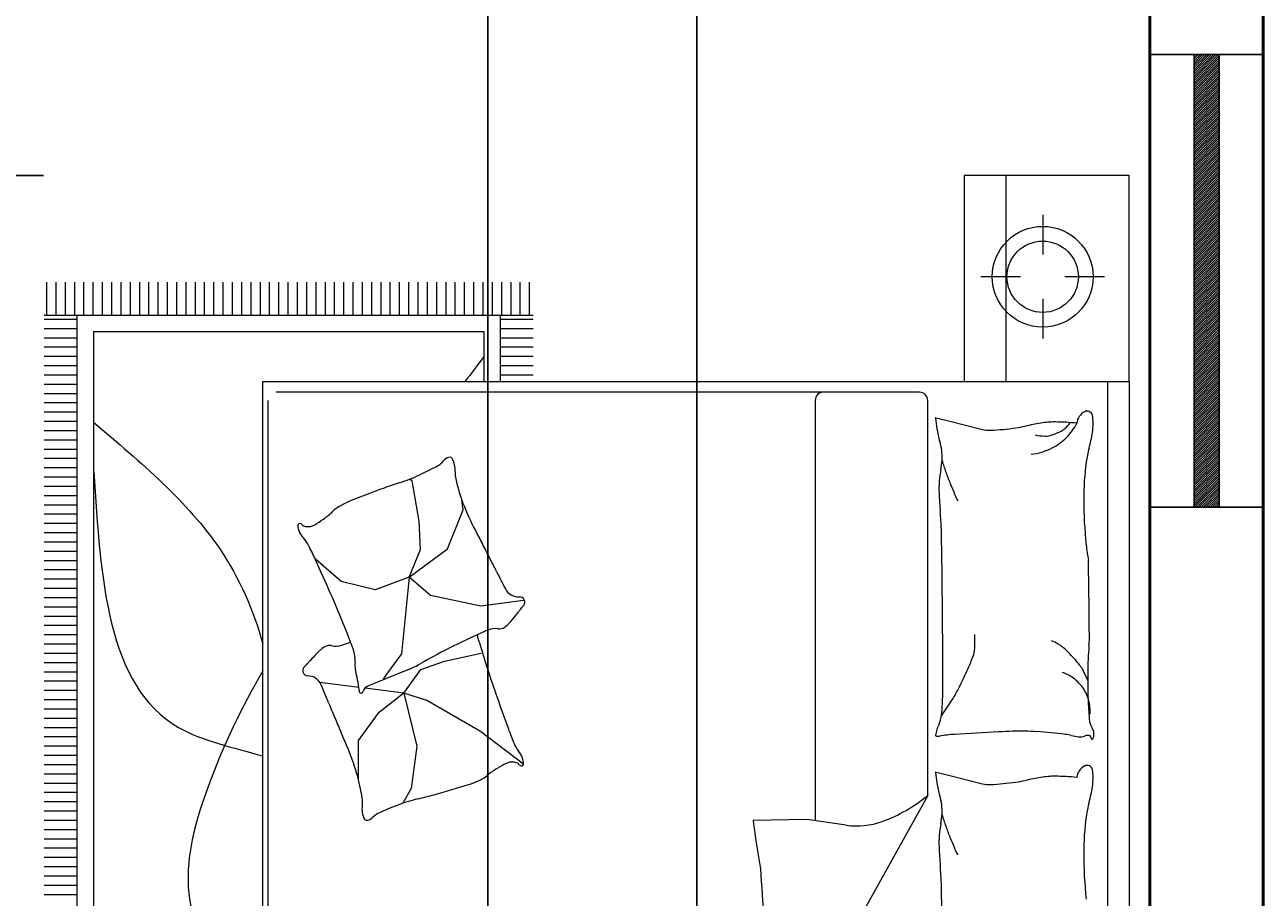
# Model space of a CAD drawing. Units: inches. Extents: x 338 to 1188, y -996 to 127.
# Tile 11 of 15: x 859 to 957, y -552 to -483. Entities that reach past the tile are written whole.
import ezdxf

# ---------------------------------------------------------------- set-up
doc = ezdxf.new("R2010")
doc.units = ezdxf.units.IN
doc.header["$MEASUREMENT"] = 0
for name, color, linetype, lineweight in [('A-ANNO-DIMS', 5, 'Continuous', 18), ('A-GLAZ-PATT', 5, 'Continuous', 13), ('wall', 1, 'Continuous', 50), ('win', 5, 'Continuous', 25)]:
    doc.layers.add(name, color=color, linetype=linetype, lineweight=lineweight)
doc.layers.add('furniture', color=50, linetype='Continuous', lineweight=13, transparency=0.8)
doc.styles.add('DIM_FONT', font='SIMPLEX.shx', dxfattribs={"width": 0.8})
doc.styles.get("Standard").update_dxf_attribs({"font": 'arial.ttf'})
doc.dimstyles.get("Standard").update_dxf_attribs({"dimtxt": 0.18, "dimasz": 0.18, "dimexe": 0.18, "dimexo": 0.0625, "dimgap": 0.09, "dimtad": 0, "dimtih": 1, "dimtoh": 1, "dimdec": 1, "dimzin": 0, "dimdsep": 46, "dimlunit": 4, "dimtxsty": 'Standard', "dimcen": 0.09, "dimadec": 0, "dimazin": 0, "dimtfac": 1, "dimtdec": 1, "dimtofl": 0, "dimtmove": 0, "dimatfit": 3, "dimfxl": 1, "dimtolj": 1, "dimtzin": 0, "dimarcsym": 0})

# ---------------------------------------------------------------- blocks, each defined once
blk = doc.blocks.new('A$C4F634EDD')
for p, q in [((0, 2.6295), (0, 2.2295)), ((0.5, 2.6295), (0, 2.6295)), ((0.5, 2.6295), (2.3, 2.6295)), ((0.5, 0.5295), (0.5, 2.6295)), ((0.5, 2.2295), (0.5, 2.6295)), ((0.2457, 2.5697), (0.2457, 2.4733)), ((0.5, 2.5771), (2.3, 2.5771)), ((0.0957, 2.4197), (0.192, 2.4197)), ((0.2994, 2.4197), (0.3957, 2.4197)), ((0.2457, 2.366), (0.2457, 2.2697)), ((0, 2.3301), (0.5, 2.3301)), ((0.5953, 2.1912), (0.616, 2.2738)), ((1.4546, 2.1912), (1.4752, 2.2738)), ((0, 2.2295), (0.5, 2.2295)), ((0.5878, 2.1612), (0.5953, 2.1912)), ((1.4471, 2.1612), (1.4546, 2.1912)), ((1.5035, 2.141), (0.5458, 2.141)), ((1.5035, 2.141), (2.2716, 1.7136)), ((0.5258, 2.121), (0.5258, 0.5617)), ((1.576, 1.9433), (1.5624, 1.8479)), ((0.5458, 1.8684), (1.5653, 1.8684)), ((1.5624, 1.8479), (1.5641, 1.7178)), ((0.2586, 1.1753), (0.3386, 1.1753)), ((0.3386, 0), (0.3386, 1.1852)), ((0.3486, 1.1052), (0.3486, 1.1852)), ((0.3711, 1.1052), (0.3711, 1.1852)), ((0.3936, 1.1052), (0.3936, 1.1852)), ((0.4161, 1.1052), (0.4161, 1.1852)), ((0.4386, 1.1052), (0.4386, 1.1852)), ((0.4611, 1.1052), (0.4611, 1.1852)), ((0.4836, 1.1052), (0.4836, 1.1852)), ((0.2586, 1.1528), (0.3386, 1.1528)), ((1.031, 1.1612), (1.0448, 1.0581)), ((1.4276, 1.1611), (1.3484, 1.0571)), ((0.2586, 1.1303), (0.3386, 1.1303)), ((0.2586, 1.1078), (0.3386, 1.1078)), ((0.2586, 1.0853), (0.3386, 1.0853)), ((0.3386, 1.1052), (0.5, 1.1052)), ((0.2586, 1.0628), (0.3386, 1.0628)), ((0.3786, 1.0652), (0.5, 1.0652)), ((0.3786, 0.12), (0.3786, 1.0652)), ((1.0448, 1.0581), (1.019, 0.936)), ((1.1784, 0.9702), (1.1586, 1.0591)), ((1.3484, 1.0571), (1.2733, 0.9268)), ((0.2586, 1.0403), (0.3386, 1.0403)), ((0.2586, 1.0178), (0.3386, 1.0178)), ((0.2586, 0.9953), (0.3386, 0.9953)), ((0.8108, 1.0151), (0.7868, 1.0117)), ((0.9054, 0.9773), (0.8108, 1.0151)), ((0.2586, 0.9728), (0.3386, 0.9728)), ((0.9743, 0.8845), (0.9054, 0.9773)), ((1.1982, 0.9129), (1.1784, 0.9702)), ((0.2586, 0.9503), (0.3386, 0.9503)), ((1.019, 0.936), (0.9743, 0.8845)), ((0.2586, 0.9278), (0.3386, 0.9278)), ((0.2586, 0.9053), (0.3386, 0.9053)), ((0.8384, 0.9085), (0.7403, 0.8913)), ((0.9072, 0.912), (0.8384, 0.9085)), ((0.9743, 0.8845), (0.9072, 0.912)), ((1.2555, 0.8715), (1.1982, 0.9129)), ((1.2733, 0.9268), (1.2555, 0.8715)), ((1.2555, 0.8715), (1.384, 0.9031)), ((1.384, 0.9031), (1.4868, 0.8892)), ((0.2586, 0.8828), (0.3386, 0.8828)), ((0.7403, 0.8913), (0.737, 0.8849)), ((0.9743, 0.8845), (1.0052, 0.802)), ((0.9743, 0.8845), (1.16, 0.8656)), ((1.1973, 0.8853), (1.2203, 0.829)), ((1.2555, 0.8715), (1.2437, 0.7773)), ((1.2555, 0.8715), (1.3049, 0.8082)), ((1.4868, 0.8892), (1.5228, 0.8692)), ((0.2586, 0.8603), (0.3386, 0.8603)), ((1.16, 0.8656), (1.2099, 0.8295)), ((0.2586, 0.8378), (0.3386, 0.8378)), ((0.2586, 0.8153), (0.3386, 0.8153)), ((1.2099, 0.8295), (1.222, 0.8209)), ((1.2203, 0.829), (1.2381, 0.7855)), ((0.2586, 0.7928), (0.3386, 0.7928)), ((1.0052, 0.802), (0.9846, 0.7194)), ((1.3049, 0.8082), (1.3701, 0.7608)), ((0.2586, 0.7703), (0.3386, 0.7703)), ((1.2419, 0.7626), (1.23, 0.668)), ((1.3701, 0.7608), (1.463, 0.7608)), ((0.2586, 0.7478), (0.3386, 0.7478)), ((0.2586, 0.7253), (0.3386, 0.7253)), ((0.2586, 0.7028), (0.3386, 0.7028)), ((0.9846, 0.7194), (0.931, 0.6569)), ((0.2586, 0.6803), (0.3386, 0.6803)), ((0.2586, 0.6578), (0.3386, 0.6578)), ((0.2586, 0.6353), (0.3386, 0.6353)), ((0.2586, 0.6128), (0.3386, 0.6128)), ((0.2586, 0.5903), (0.3386, 0.5903)), ((0.2586, 0.5678), (0.3386, 0.5678)), ((0.2586, 0.5453), (0.3386, 0.5453)), ((0.5458, 0.5417), (2.2516, 0.5417)), ((0.2586, 0.5228), (0.3386, 0.5228)), ((2.3, 0.5295), (0.5, 0.5295)), ((0.2586, 0.5003), (0.3386, 0.5003)), ((0.2586, 0.4778), (0.3386, 0.4778)), ((0.2586, 0.4553), (0.3386, 0.4553)), ((0.2586, 0.4328), (0.3386, 0.4328)), ((0.2586, 0.4103), (0.3386, 0.4103)), ((0.2586, 0.3878), (0.3386, 0.3878)), ((0.2586, 0.3653), (0.3386, 0.3653)), ((0.2586, 0.3428), (0.3386, 0.3428)), ((0.2586, 0.3203), (0.3386, 0.3203)), ((0.2586, 0.2978), (0.3386, 0.2978)), ((0.2586, 0.2753), (0.3386, 0.2753)), ((0.2586, 0.2528), (0.3386, 0.2528)), ((0.2586, 0.2303), (0.3386, 0.2303)), ((0.2586, 0.2078), (0.3386, 0.2078)), ((0.2586, 0.1853), (0.3386, 0.1853)), ((0.2586, 0.1628), (0.3386, 0.1628)), ((0.2586, 0.1403), (0.3386, 0.1403)), ((0.2586, 0.1178), (0.3386, 0.1178)), ((0.2586, 0.0953), (0.3386, 0.0953)), ((2.4188, 0.12), (0.3786, 0.12)), ((0.2586, 0.0728), (0.3386, 0.0728)), ((2.4588, 0.08), (0.3386, 0.08)), ((0.3486, 0), (0.3486, 0.08)), ((0.3711, 0), (0.3711, 0.08)), ((0.3936, 0), (0.3936, 0.08)), ((0.4161, 0), (0.4161, 0.08)), ((0.4386, 0), (0.4386, 0.08)), ((0.4611, 0), (0.4611, 0.08)), ((0.4836, 0), (0.4836, 0.08)), ((0.5061, 0), (0.5061, 0.08)), ((0.5286, 0), (0.5286, 0.08)), ((0.5511, 0), (0.5511, 0.08)), ((0.5736, 0), (0.5736, 0.08)), ((0.5961, 0), (0.5961, 0.08)), ((0.6186, 0), (0.6186, 0.08)), ((0.6411, 0), (0.6411, 0.08)), ((0.6636, 0), (0.6636, 0.08)), ((0.6861, 0), (0.6861, 0.08)), ((0.7086, 0), (0.7086, 0.08)), ((0.7311, 0), (0.7311, 0.08)), ((0.7536, 0), (0.7536, 0.08)), ((0.7761, 0), (0.7761, 0.08)), ((0.7986, 0), (0.7986, 0.08)), ((0.8211, 0), (0.8211, 0.08)), ((0.8436, 0), (0.8436, 0.08)), ((0.8661, 0), (0.8661, 0.08)), ((0.8886, 0), (0.8886, 0.08)), ((0.9111, 0), (0.9111, 0.08)), ((0.9336, 0), (0.9336, 0.08)), ((0.9561, 0), (0.9561, 0.08)), ((0.9786, 0), (0.9786, 0.08)), ((1.0011, 0), (1.0011, 0.08)), ((1.0236, 0), (1.0236, 0.08)), ((1.0461, 0), (1.0461, 0.08)), ((1.0686, 0), (1.0686, 0.08)), ((1.0911, 0), (1.0911, 0.08)), ((1.1136, 0), (1.1136, 0.08)), ((1.1361, 0), (1.1361, 0.08)), ((1.1586, 0), (1.1586, 0.08)), ((1.1811, 0), (1.1811, 0.08)), ((1.2036, 0), (1.2036, 0.08)), ((1.2261, 0), (1.2261, 0.08)), ((1.2486, 0), (1.2486, 0.08)), ((1.2711, 0), (1.2711, 0.08)), ((1.2936, 0), (1.2936, 0.08)), ((1.3161, 0), (1.3161, 0.08)), ((1.3386, 0), (1.3386, 0.08)), ((1.3611, 0), (1.3611, 0.08)), ((1.3836, 0), (1.3836, 0.08)), ((1.4061, 0), (1.4061, 0.08)), ((1.4286, 0), (1.4286, 0.08)), ((1.4511, 0), (1.4511, 0.08)), ((1.4736, 0), (1.4736, 0.08)), ((1.4961, 0), (1.4961, 0.08)), ((1.5186, 0), (1.5186, 0.08)), ((1.5411, 0), (1.5411, 0.08)), ((1.5636, 0), (1.5636, 0.08)), ((1.5861, 0), (1.5861, 0.08)), ((1.6086, 0), (1.6086, 0.08)), ((1.6311, 0), (1.6311, 0.08)), ((1.6536, 0), (1.6536, 0.08)), ((1.6761, 0), (1.6761, 0.08)), ((1.6986, 0), (1.6986, 0.08)), ((1.7211, 0), (1.7211, 0.08)), ((1.7436, 0), (1.7436, 0.08)), ((0.2586, 0.0503), (0.3386, 0.0503)), ((0.2586, 0.0278), (0.3386, 0.0278)), ((0.2586, 0.0053), (0.3386, 0.0053))]:
    blk.add_line(p, q)
for radius in [0.1222, 0.0865]:
    blk.add_circle((0.2457, 2.4197), radius)
for centre, radius, start, end in [((0.5848, 2.5274), 0.0131, 101.2724, 206.5805), ((0.6036, 2.5368), 0.0342, 206.5805, 265.5998), ((0.5999, 2.4516), 0.0904, 90, 101.2724), ((0.5999, 2.3808), 0.1611, 81.5628, 90), ((0.5788, 2.2388), 0.3048, 74.256, 81.5628), ((0.7272, 2.7653), 0.2422, 254.256, 262.4531), ((0.7851, 3.2019), 0.6827, 262.4531, 270), ((0.7851, 3.5682), 1.049, 270, 276.0867), ((0.8402, 3.0514), 0.5293, 276.0867, 280.1899), ((1.1602, -8.1346), 10.6675, 90.30153, 91.21582), ((1.1169, 2.2433), 0.2897, 85.1982, 92.5386), ((1.2142, 3.4021), 0.8732, 265.1982, 269.4243), ((1.3082, 2.3102), 0.234, 110.8603, 117.2396), ((1.2204, 4.0232), 1.4943, 269.4243, 271.9079), ((1.2995, 2.4357), 0.0992, 105.9352, 126.0864), ((1.2429, 3.3501), 0.8208, 271.9079, 275.2592), ((1.2995, 2.4357), 0.0992, 85.7841, 105.9352), ((1.3132, 2.5864), 0.0539, 275.2592, 300.6513), ((1.3554, 2.5152), 0.0289, 85.6975, 120.6513), ((1.3556, 2.519), 0.0251, 68.2117, 85.6975), ((1.3739, 2.5288), 0.0156, 158.0096, 201.421), ((1.3634, 2.533), 0.00428, 78.1069, 158.0096), ((1.3288, 2.5111), 0.0328, 351.8665, 21.421), ((1.3647, 2.5395), 0.00232, 258.1069, 19.564), ((1.3637, 2.5391), 0.00342, 19.564, 68.2117), ((1.444, 2.5274), 0.0131, 101.2724, 206.5805), ((1.4628, 2.5368), 0.0342, 206.5805, 265.5998), ((1.4591, 2.4516), 0.0904, 90, 101.2724), ((1.4591, 2.3808), 0.1611, 81.5628, 90), ((1.438, 2.2388), 0.3048, 74.256, 81.5628), ((1.5865, 2.7653), 0.2422, 254.256, 262.4531), ((1.6443, 3.2019), 0.6827, 262.4531, 270), ((1.6443, 3.5682), 1.049, 270, 276.0867), ((1.0898, 2.4496), 0.4918, 173.7676, 180), ((0.5368, 2.3783), 0.1399, 45.0976, 62.7964), ((1.4317, 2.2032), 0.3916, 128.3886, 133.8115), ((1.2362, 2.45), 0.0768, 117.2396, 128.3886), ((1.2995, 2.4357), 0.0992, 143.8234, 161.5603), ((1.2995, 2.4357), 0.0992, 126.0864, 143.8234), ((1.1177, 2.5413), 0.246, 347.8905, 351.8665), ((1.949, 2.4496), 0.4918, 173.7676, 180), ((0.5462, 2.4142), 0.0899, 41.4429, 53.7359), ((0.5741, 2.4389), 0.0526, 25.3551, 41.4429), ((0.4851, 2.3967), 0.1511, 21.8149, 25.3551), ((0.5368, 2.3783), 0.1399, 27.3988, 45.0976), ((1.1799, 2.4341), 0.0493, 140.9651, 151.6832), ((1.3165, 2.3233), 0.2252, 133.8115, 140.9651), ((2.2605, 2.3525), 0.9131, 172.3191, 176.6313), ((1.5522, 2.448), 0.1983, 167.8905, 172.3191), ((0.8019, 2.4496), 0.204, 180, 189.6844), ((0.4345, 2.3765), 0.2056, 18.7799, 21.8149), ((0.576, 2.4246), 0.0562, 0, 18.7799), ((0.5368, 2.3783), 0.1399, 16.515, 27.3988), ((1.3127, 2.3625), 0.2002, 151.6832, 156.9972), ((1.6611, 2.4496), 0.204, 180, 189.6844), ((1.4703, 2.5637), 0.882, 189.6844, 192.1984), ((0.5406, 2.4246), 0.0915, 345.3149, 0), ((0.5368, 2.3783), 0.1399, 5.6311, 16.515), ((2.0266, 2.3663), 0.6787, 176.6313, 181.6331), ((2.3295, 2.5637), 0.882, 189.6844, 192.1984), ((0.2982, 2.3103), 0.3171, 8.0051, 12.1984), ((1.1575, 2.3103), 0.3171, 8.0051, 12.1984), ((-0.0401, 2.2627), 0.6588, 2.6649, 8.0051), ((2.7128, 2.3859), 1.3652, 181.6331, 183.055), ((0.8191, 2.2627), 0.6588, 2.6649, 8.0051), ((14.9657, 3.0398), 13.6356, 183.05496, 183.50486), ((0.5503, 2.2902), 0.0677, 345.9548, 2.6649), ((1.4096, 2.2902), 0.0677, 345.9548, 2.6649), ((1.1303, 1.9835), 0.2721, 85.9172, 93.5552), ((1.1455, 2.197), 0.058, 69.3257, 85.9172), ((0.9871, 1.7772), 0.5066, 65.6735, 69.3257), ((0.6058, 0.9338), 1.4323, 63.5015, 65.6735), ((0.473, 2.8815), 0.7387, 289.428, 291.6577), ((0.473, 2.8815), 0.7387, 291.6577, 293.4844), ((0.473, 2.8815), 0.7387, 293.4844, 295.3111), ((1.1054, 1.9358), 0.3126, 57.865, 63.5015), ((0.8841, 1.5835), 0.7286, 54.1737, 57.865), ((1.6762, 2.2258), 0.3212, 183.5049, 189.9984), ((1.3322, 2.8815), 0.7387, 289.428, 291.6577), ((1.3322, 2.8815), 0.7387, 291.6577, 293.4844), ((1.3322, 2.8815), 0.7387, 293.4844, 295.3111), ((0.5695, 2.4301), 0.2708, 274.0829, 279.4841), ((0.5763, 2.3896), 0.2297, 279.4841, 287.3864), ((0.6807, 2.0561), 0.1197, 96.4341, 107.3864), ((0.6836, 2.0301), 0.1459, 78.4414, 96.4341), ((0.473, 2.8815), 0.7387, 287.1982, 289.428), ((0.759, 2.3985), 0.2301, 258.4414, 272.7491), ((0.7026, 3.5718), 1.4048, 272.7491, 274.6176), ((0.9136, 0.9591), 1.2165, 92.6096, 94.6176), ((1.2501, -19.8405), 22.0183, 90.37908, 91.01965), ((1.2012, -3.5404), 5.7185, 89.7135, 90.9704), ((1.224, 1.0141), 1.164, 86.426, 89.7135), ((1.2875, 2.0302), 0.1459, 77.131, 86.426), ((1.3099, 2.1283), 0.0453, 62.7159, 77.131), ((1.3658, 2.2367), 0.0767, 242.7159, 253.7788), ((1.3688, 2.247), 0.0875, 253.7788, 262.8796), ((1.3409, 2.1667), 0.0193, 343.3022, 9.9984), ((1.4288, 2.4301), 0.2708, 274.0829, 279.4841), ((1.4355, 2.3896), 0.2297, 279.4841, 287.3864), ((1.5399, 2.0561), 0.1197, 96.4341, 107.3864), ((1.5429, 2.0301), 0.1459, 78.4414, 96.4341), ((1.3322, 2.8815), 0.7387, 287.1982, 289.428), ((1.6182, 2.3985), 0.2301, 258.4414, 272.7491), ((1.5619, 3.5718), 1.4048, 272.7491, 274.6176), ((1.7729, 0.9591), 1.2165, 92.6096, 94.6176), ((2.1093, -19.8405), 22.0183, 90.37908, 91.01965), ((0.5458, 2.121), 0.02, 90, 180), ((0.5887, 2.1609), 0.000917, 165.9551, 274.0829), ((1.3581, 2.1615), 0.00132, 262.8796, 343.3022), ((1.448, 2.1609), 0.000917, 165.9551, 274.0829), ((1.2147, 1.9017), 0.3751, 20.1488, 39.6445), ((1.3977, 1.9688), 0.1801, 351.8644, 20.1488), ((0.5458, 1.8884), 0.02, 180, 270), ((0.6102, 18.0525), 16.3521, 273.75703, 274.62393), ((1.0582, 5.4638), 3.7801, 277.692, 279.495), ((0.9863, 1.1494), 0.0359, 297.2902, 3.2455), ((1.0348, 1.1521), 0.0127, 51.1864, 183.2455), ((0.9991, 1.1077), 0.0697, 45.8726, 51.1864), ((1.0791, 1.1902), 0.0452, 225.8726, 232.4713), ((1.2846, 1.4577), 0.3825, 232.4713, 233.7837), ((0.6683, 0.6162), 0.6605, 52.7849, 53.7837), ((0.9362, 0.9689), 0.2176, 46.4776, 52.7849), ((1.3469, 1.2115), 0.0792, 292.7069, 308.5854), ((1.4338, 1.1026), 0.0601, 110.3452, 128.5854), ((1.4251, 1.1259), 0.0352, 86.0516, 110.3452), ((1.4996, 1.1284), 0.0771, 169.5926, 177.2714), ((1.4376, 1.1398), 0.0142, 126.5792, 169.5926), ((1.4273, 1.1567), 0.00443, 13.2808, 86.0516), ((1.4254, 1.1562), 0.0063, 306.5792, 13.2808), ((-0.4173, 3.8699), 3.0972, 296.4147, 297.2902), ((1.0327, 1.0706), 0.0774, 35.8936, 46.4776), ((1.0771, 1.1027), 0.0226, 351.9508, 35.8936), ((-0.4107, 5.9078), 5.0942, 289.0836, 290.1287), ((1.0543, 1.9106), 0.8371, 290.1287, 292.7069), ((1.4378, 1.1314), 0.0153, 177.2714, 194.5709), ((1.4611, 1.1374), 0.0393, 194.5709, 206.8179), ((1.7401, 1.2785), 0.352, 206.8179, 210.9056), ((1.8575, -0.7096), 2.0162, 116.4147, 117.4999), ((1.1449, 1.0931), 0.0458, 171.9508, 202.4162), ((0.2266, 4.0657), 3.145, 286.6085, 289.0836), ((1.6045, 1.1973), 0.194, 210.9056, 219.7005), ((-1.8336, 6.2238), 5.8383, 297.49208, 297.84822), ((3.744, -4.3336), 6.1019, 117.49986, 117.84822), ((2.032, 1.4591), 1.0054, 202.4162, 205.0529), ((1.0922, 1.1636), 0.1166, 280.7366, 286.6085), ((1.3929, 1.0217), 0.081, 26.0735, 39.7005), ((1.2892, 0.9709), 0.1965, 17.8396, 26.0735), ((0.5736, 1.5979), 0.6236, 290.7486, 297.4921), ((2.6493, 1.7476), 1.6868, 205.0529, 207.0884), ((-0.4304, 0.4175), 2.003, 15.2625, 17.8396), ((0.7131, 0.9448), 0.0509, 103.0402, 121.6917), ((0.7152, 0.9361), 0.0599, 86.6119, 103.0402), ((0.7224, 1.0587), 0.063, 266.6119, 282.6252), ((0.6422, 1.4168), 0.43, 282.6252, 290.7486), ((0.6894, 0.9832), 0.0058, 121.6917, 179.0386), ((0.7004, 0.983), 0.0168, 179.0386, 229.4914), ((0.6405, 0.9128), 0.0755, 26.3332, 49.4914), ((2.541, 1.6922), 1.5652, 207.0884, 209.936), ((-1.6775, -0.2344), 2.6619, 25.1732, 26.3332), ((-0.0881, 0.5109), 1.6481, 13.841, 15.2625), ((0.9989, 0.8042), 0.2143, 22.2355, 29.936), ((2.0418, 1.0357), 0.5454, 193.841, 196.3122), ((0.5689, 0.8213), 0.1798, 20.7081, 25.1732), ((0.2268, 0.692), 0.5454, 18.2369, 20.7081), ((1.6908, 0.933), 0.1798, 196.3122, 200.7773), ((2.3102, 1.3785), 1.6481, 198.2369, 199.6584), ((4.0115, 1.8135), 2.6619, 200.7773, 201.9373), ((2.6444, 1.4979), 2.003, 199.6584, 202.2355), ((1.6124, 0.8472), 0.0755, 201.9373, 225.0955), ((1.2594, 0.7942), 0.0231, 202.2355, 252.8133), ((1.5473, 0.7819), 0.0168, 354.6428, 45.0955), ((1.1834, 0.6373), 0.1166, 98.1216, 111.0043), ((1.1763, 0.687), 0.0663, 85.4882, 98.1216), ((1.1871, 0.8241), 0.0712, 265.4882, 277.6784), ((1.1727, 0.9313), 0.1794, 277.6784, 284.8807), ((1.2689, 0.569), 0.1955, 97.9822, 104.8807), ((1.2465, 0.729), 0.034, 85.7407, 97.9822), ((1.2497, 0.772), 0.0092, 265.7407, 289.3799), ((1.2512, 0.7678), 0.00467, 289.3799, 72.8133), ((1.6266, 0.159), 0.6236, 106.3527, 113.0962), ((1.5721, 0.3449), 0.43, 98.2293, 106.3527), ((1.5195, 0.708), 0.063, 82.216, 98.2293), ((1.5362, 0.8298), 0.0599, 262.216, 278.6443), ((1.5375, 0.8209), 0.0509, 278.6443, 297.2959), ((1.5582, 0.7808), 0.0058, 297.2959, 354.6428), ((0.9722, 0.8143), 0.1965, 202.2355, 210.4694), ((2.2689, -2.1899), 3.145, 111.0043, 113.4795), ((0.1831, 0.4093), 1.0054, 18.0203, 19.3448), ((3.6722, -4.6377), 5.8383, 113.0962, 113.45234), ((0.8727, 0.7557), 0.081, 210.4694, 224.0964), ((0.6752, 0.5644), 0.194, 35.3015, 44.0964), ((3.0455, -3.9778), 5.0942, 113.4795, 114.5246), ((1.0957, 0.7061), 0.0458, 347.5549, 18.0203), ((1.1625, 0.6914), 0.0226, 167.5549, 211.4977), ((0.5234, 2.5582), 2.0162, 292.0188, 293.104), ((-1.0798, 6.3161), 6.1019, 293.10398, 293.45234), ((0.5462, 0.4731), 0.352, 31.2138, 35.3015), ((1.2092, 0.72), 0.0774, 211.4977, 222.0817), ((1.3133, 0.814), 0.2176, 222.0817, 228.389), ((1.2495, 0.6379), 0.0359, 112.8944, 178.8496), ((2.4404, -2.1823), 3.0972, 112.0188, 112.8944), ((0.8372, 0.6345), 0.0142, 310.9751, 353.9885), ((0.8136, 0.6351), 0.0393, 18.9668, 31.2138), ((0.8364, 0.6429), 0.0153, 1.6673, 18.9668), ((0.7746, 0.6411), 0.0771, 353.9885, 1.6673), ((0.9332, 0.57), 0.0792, 117.1028, 132.9813), ((1.2784, -0.1047), 0.8371, 114.5246, 117.1028), ((1.6074, 1.1451), 0.6605, 228.389, 229.3878), ((0.9284, 0.3533), 0.3825, 48.0754, 49.3878), ((1.1538, 0.6043), 0.0452, 41.4767, 48.0754), ((1.2399, 0.6804), 0.0697, 221.4767, 226.7905), ((1.2009, 0.6389), 0.0127, 226.7905, 358.8496), ((0.8506, 0.6191), 0.0063, 130.9751, 197.6767), ((0.8488, 0.6185), 0.00443, 197.6767, 270.4475), ((0.8486, 0.6493), 0.0352, 270.4475, 294.7411), ((0.8382, 0.6719), 0.0601, 294.7411, 312.9813)]:
    blk.add_arc(centre, radius, start, end)
blk.add_open_spline([(0.4393, 1.0652), (0.4595, 1.05), (0.4798, 1.0348), (0.5, 1.0195)], degree=3)
for points, knots in [([(0.5992, 0.12), (0.6957, 0.2341), (0.8523, 0.4189), (1.0536, 0.5069), (1.136, 0.5295)], [0, 0, 0, 0, 432.822832, 701.445452, 701.445452, 701.445452, 701.445452]), ([(0.7187, 0.12), (0.9791, 0.1362), (1.326, 0.1577), (1.3868, 0.4574), (1.408, 0.5295)], [0, 0, 0, 0, 653.160442, 870.050857, 870.050857, 870.050857, 870.050857]), ([(1.2016, 0.5295), (1.2892, 0.479), (1.5144, 0.3684), (1.8265, 0.2994), (1.9681, 0.4992), (1.9875, 0.5295)], [936.534237, 936.534237, 936.534237, 936.534237, 1243.285375, 1683.261222, 1758.254386, 1758.254386, 1758.254386, 1758.254386])]:
    blk.add_open_spline(points, degree=3, knots=knots)
at = {"style": 'DIM_FONT', "width": 0.8, "flags": 9}
for tag, p in [('YSIZE', (0.5, 2.6295)), ('XSIZE', (0.5, 2.6295)), ('XSIZE', (2.2985, 2.6295)), ('YSIZE', (2.2985, 2.6295))]:
    blk.add_attdef(tag, p, '', height=0.0005, dxfattribs=at)
blk = doc.blocks.new('*D19')
at = {"layer": 'A-ANNO-DIMS', "color": 0, "lineweight": -2, "transparency": 16777216}
for p, q in [((860.056, -494.839), (846.17, -494.839)), ((846.35, -495.019), (846.35, -540.551)), ((846.35, -586.447), (846.35, -540.915)), ((860.056, -586.627), (846.17, -586.627))]:
    blk.add_line(p, q, dxfattribs=at)
at = {"layer": 'A-ANNO-DIMS', "color": 0, "transparency": 16777216}
for points in [[(846.32, -495.019), (846.38, -495.019), (846.35, -494.839)], [(846.32, -586.447), (846.38, -586.447), (846.35, -586.627)]]:
    blk.add_solid(points, dxfattribs=at)
at = {"layer": 'Defpoints', "color": 0, "transparency": 16777216}
for p in [(860.118, -494.839), (846.35, -586.627), (860.118, -586.627)]:
    blk.add_point(p, dxfattribs=at)
at = {"layer": 'A-ANNO-DIMS', "color": 0, "transparency": 16777216, "insert": (846.35, -540.733), "char_height": 0.18, "attachment_point": 5}
blk.add_mtext('\\A1;BED 7\'-8"', dxfattribs=at)
blk = doc.blocks.new('*D27')
at = {"layer": 'A-ANNO-DIMS', "color": 0, "lineweight": -2, "transparency": 16777216}
for p, q in [((911.963, -297.796), (911.963, -968.856)), ((947.963, -297.796), (947.963, -968.856)), ((912.143, -968.676), (929.634, -968.676)), ((947.783, -968.676), (930.292, -968.676))]:
    blk.add_line(p, q, dxfattribs=at)
at = {"layer": 'A-ANNO-DIMS', "color": 0, "transparency": 16777216}
for points in [[(912.143, -968.646), (912.143, -968.706), (911.963, -968.676)], [(947.783, -968.646), (947.783, -968.706), (947.963, -968.676)]]:
    blk.add_solid(points, dxfattribs=at)
at = {"layer": 'Defpoints', "color": 0, "transparency": 16777216}
for p in [(911.963, -297.733), (947.963, -297.733), (947.963, -968.676)]:
    blk.add_point(p, dxfattribs=at)
at = {"layer": 'A-ANNO-DIMS', "color": 0, "transparency": 16777216, "insert": (929.963, -968.676), "char_height": 0.18, "attachment_point": 5}
blk.add_mtext('\\A1;3\'-0"', dxfattribs=at)
blk = doc.blocks.new('*D28')
at = {"layer": 'A-ANNO-DIMS', "color": 0, "lineweight": -2, "transparency": 16777216}
for p, q in [((803.963, -265.796), (803.963, -968.856)), ((947.963, -297.796), (947.963, -968.856)), ((804.143, -968.676), (875.573, -968.676)), ((947.783, -968.676), (876.354, -968.676))]:
    blk.add_line(p, q, dxfattribs=at)
at = {"layer": 'A-ANNO-DIMS', "color": 0, "transparency": 16777216}
for points in [[(804.143, -968.646), (804.143, -968.706), (803.963, -968.676)], [(947.783, -968.646), (947.783, -968.706), (947.963, -968.676)]]:
    blk.add_solid(points, dxfattribs=at)
at = {"layer": 'Defpoints', "color": 0, "transparency": 16777216}
for p in [(803.963, -265.733), (947.963, -297.733), (947.963, -968.676)]:
    blk.add_point(p, dxfattribs=at)
at = {"layer": 'A-ANNO-DIMS', "color": 0, "transparency": 16777216, "insert": (875.963, -968.676), "char_height": 0.18, "attachment_point": 5}
blk.add_mtext('\\A1;12\'-0"', dxfattribs=at)
blk = doc.blocks.new('*D43')
at = {"layer": 'A-ANNO-DIMS', "color": 0, "lineweight": -2, "transparency": 16777216}
for p, q in [((853.279, -53.934), (853.279, -968.856)), ((895.369, -53.934), (895.369, -968.856)), ((853.459, -968.676), (873.995, -968.676)), ((895.189, -968.676), (874.653, -968.676))]:
    blk.add_line(p, q, dxfattribs=at)
at = {"layer": 'A-ANNO-DIMS', "color": 0, "transparency": 16777216}
for points in [[(853.459, -968.646), (853.459, -968.706), (853.279, -968.676)], [(895.189, -968.646), (895.189, -968.706), (895.369, -968.676)]]:
    blk.add_solid(points, dxfattribs=at)
at = {"layer": 'Defpoints', "color": 0, "transparency": 16777216}
for p in [(853.279, -53.872), (895.369, -53.872), (895.369, -968.676)]:
    blk.add_point(p, dxfattribs=at)
at = {"layer": 'A-ANNO-DIMS', "color": 0, "transparency": 16777216, "insert": (874.324, -968.676), "char_height": 0.18, "attachment_point": 5}
blk.add_mtext('\\A1;3\'-6"', dxfattribs=at)
blk = doc.blocks.new('*D44')
at = {"layer": 'A-ANNO-DIMS', "color": 0, "lineweight": -2, "transparency": 16777216}
for p, q in [((895.369, -53.934), (895.369, -968.856)), ((947.963, -54.796), (947.963, -968.856)), ((895.549, -968.676), (921.124, -968.676)), ((947.783, -968.676), (922.209, -968.676))]:
    blk.add_line(p, q, dxfattribs=at)
at = {"layer": 'A-ANNO-DIMS', "color": 0, "transparency": 16777216}
for points in [[(895.549, -968.646), (895.549, -968.706), (895.369, -968.676)], [(947.783, -968.646), (947.783, -968.706), (947.963, -968.676)]]:
    blk.add_solid(points, dxfattribs=at)
at = {"layer": 'Defpoints', "color": 0, "transparency": 16777216}
for p in [(895.369, -53.872), (947.963, -54.733), (947.963, -968.676)]:
    blk.add_point(p, dxfattribs=at)
at = {"layer": 'A-ANNO-DIMS', "color": 0, "transparency": 16777216, "insert": (921.666, -968.676), "char_height": 0.18, "attachment_point": 5}
blk.add_mtext('\\A1;4\'-4 1/2"', dxfattribs=at)
blk = doc.blocks.new('*D47')
at = {"layer": 'A-ANNO-DIMS', "color": 0, "lineweight": -2, "transparency": 16777216}
for p, q in [((759.673, -755.171), (759.673, 67.247)), ((759.853, 67.067), (867.678, 67.067)), ((976.283, 67.067), (868.459, 67.067)), ((976.463, -755.171), (976.463, 67.247))]:
    blk.add_line(p, q, dxfattribs=at)
at = {"layer": 'A-ANNO-DIMS', "color": 0, "transparency": 16777216}
for points in [[(759.853, 67.097), (759.853, 67.037), (759.673, 67.067)], [(976.283, 67.097), (976.283, 67.037), (976.463, 67.067)]]:
    blk.add_solid(points, dxfattribs=at)
at = {"layer": 'Defpoints', "color": 0, "transparency": 16777216}
for p in [(976.463, 67.067), (759.673, -755.233), (976.463, -755.233)]:
    blk.add_point(p, dxfattribs=at)
at = {"layer": 'A-ANNO-DIMS', "color": 0, "transparency": 16777216, "insert": (868.068, 67.067), "char_height": 0.18, "attachment_point": 5}
blk.add_mtext('\\A1;18\'-1"', dxfattribs=at)

msp = doc.modelspace()

# ---------------------------------------------------------------- hatches: boundary and pattern name
at = {"layer": 'A-GLAZ-PATT'}
h = msp.add_hatch(dxfattribs=at)
h.set_pattern_fill('ANSI31', color=256)
h.paths.add_polyline_path([(953.463, -405.073), (951.463, -405.073), (951.463, -429.073), (953.463, -429.073)])
h.paths.add_polyline_path([(953.463, -485.222), (951.463, -485.222), (951.463, -521.222), (953.463, -521.222)])
h.paths.add_polyline_path([(794.207, -19.233), (758.207, -19.233), (758.207, -21.233), (794.207, -21.233)])
h.paths.add_polyline_path([(668.695, -19.233), (632.695, -19.233), (632.695, -21.233), (668.695, -21.233)])
h.paths.add_polyline_path([(602.463, -94.886), (600.463, -94.886), (600.463, -130.886), (602.463, -130.886)])
h.paths.add_polyline_path([(602.463, -243.733), (600.463, -243.733), (600.463, -315.733), (602.463, -315.733)])

# ---------------------------------------------------------------- linework, layer by layer
at = {"layer": 'wall'}
for p, q in [((956.963, -15.733), (956.963, -615.733)), ((947.963, -474.733), (947.963, -606.733))]:
    msp.add_line(p, q, dxfattribs=at)
at = {"layer": 'win'}
for p, q in [((947.963, -485.222), (956.963, -485.222)), ((951.463, -485.222), (951.463, -521.222)), ((953.463, -485.222), (953.463, -521.222)), ((947.963, -521.222), (956.963, -521.222))]:
    msp.add_line(p, q, dxfattribs=at)

# ---------------------------------------------------------------- block references
at = {"layer": 'furniture', "xscale": 32.78135669785699, "yscale": 32.78135669785699, "zscale": 32.78135669785699, "rotation": 270}
msp.add_blockref('A$C4F634EDD', (860.118, -494.839), dxfattribs=at)

# ---------------------------------------------------------------- dimensions: what is measured, and where the dimension line sits
at = {"layer": 'A-ANNO-DIMS'}
for base, p1, p2, picture, middle in [((976.463, 67.067), (759.673, -755.233), (976.463, -755.233), '*D47', (868.068, 67.067)), ((895.369, -968.676), (853.279, -53.872), (895.369, -53.872), '*D43', (874.324, -968.676)), ((947.963, -968.676), (895.369, -53.872), (947.963, -54.733), '*D44', (921.666, -968.676)), ((947.963, -968.676), (803.963, -265.733), (947.963, -297.733), '*D28', (875.963, -968.676)), ((947.963, -968.676), (911.963, -297.733), (947.963, -297.733), '*D27', (929.963, -968.676))]:
    dim = msp.add_linear_dim(base=base, p1=p1, p2=p2, dimstyle='Standard', override={"dimdec": 1, "dimlfac": 1, "dimrnd": 0, "dimzin": 1, "dimdsep": 46, "dimlunit": 4, "dimfrac": 2}, dxfattribs=at)
    dim.commit()
    dim.dimension.update_dxf_attribs({"geometry": picture, "text_midpoint": middle})
dim = msp.add_linear_dim(base=(846.35, -586.627), p1=(860.118, -494.839), p2=(860.118, -586.627), angle=270, text='BED <>', dimstyle='Standard', override={"dimdec": 1, "dimlfac": 1, "dimrnd": 0, "dimzin": 1, "dimdsep": 46, "dimlunit": 4, "dimfrac": 2}, dxfattribs=at)
dim.commit()
dim.dimension.update_dxf_attribs({"geometry": '*D19', "text_midpoint": (846.35, -540.733)})

doc.saveas('drawing.dxf')
